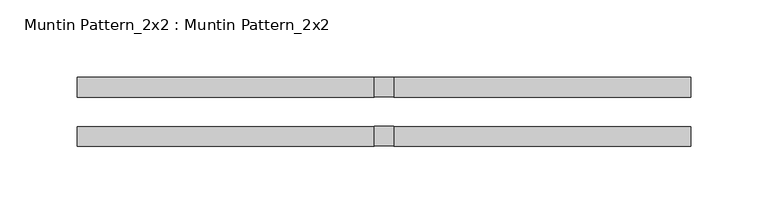
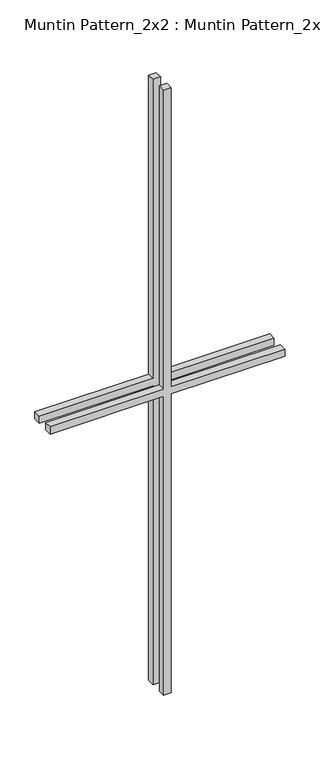
"""IFC4 building model written with IfcOpenShell, lengths in millimetres: proxy geometry, Muntin Pattern_2x2 : Muntin Pattern_2x2."""

from ifc_helpers import new_model, si_unit, frame, origin, place, context, project, spatial, polyline, outline, extrude, source, transform, mapped, element, save


def muntin_pattern_2x2_muntin_pattern_2x2_63e5058f(model_context):
    return source(origin(), model_context, "Body", "SweptSolid", [
        extrude(outline(polyline([(546.1, -6.35), (546.1, -198.4375), (533.4, -198.4375), (533.4, -6.35), (0.0, -6.35), (0.0, 6.35), (533.4, 6.35), (533.4, 198.4375), (546.1, 198.4375), (546.1, 6.35), (1079.5, 6.35), (1079.5, -6.35), (546.1, -6.35)])), frame((0.0, 9.525, 0.0), z_axis=(0.0, 1.0, 0.0), x_axis=(0.0, 0.0, 1.0)), (0.0, 0.0, 1.0), 12.7),
        extrude(outline(polyline([(546.1, -6.35), (546.1, -198.4375), (533.4, -198.4375), (533.4, -6.35), (0.0, -6.35), (0.0, 6.35), (533.4, 6.35), (533.4, 198.4375), (546.1, 198.4375), (546.1, 6.35), (1079.5, 6.35), (1079.5, -6.35), (546.1, -6.35)])), frame((0.0, -22.225, 0.0), z_axis=(0.0, 1.0, 0.0), x_axis=(0.0, 0.0, 1.0)), (0.0, 0.0, 1.0), 12.7),
    ])


if __name__ == "__main__":
    model = new_model("IFC4")
    model_context = context("Model", 3, world=origin())
    ifc_project = project(units=[si_unit("LENGTHUNIT", "METRE", prefix="MILLI")], contexts=[model_context])
    site = spatial("IfcSite", under=ifc_project)
    building = spatial("IfcBuilding", under=site)
    placement = place(None, origin())
    muntin_pattern_2x2_muntin_pattern_2x2_shape = muntin_pattern_2x2_muntin_pattern_2x2_63e5058f(model_context)
    element("IfcBuildingElementProxy", 1, Name="Muntin Pattern_2x2 : Muntin Pattern_2x2", ObjectType="Muntin Pattern_2x2 : Muntin Pattern_2x2", at=placement, inside=building, context=model_context, shape_type="MappedRepresentation", body=[
        mapped(muntin_pattern_2x2_muntin_pattern_2x2_shape, transform((0.0, 0.0, 0.0), x_axis=(1.0, 0.0, 0.0), y_axis=(0.0, 1.0, 0.0), z_axis=(0.0, 0.0, 1.0))),
    ])
    save(model, "model.ifc")

# Revit data of these elements
# Type "Muntin Pattern_2x2 : Muntin Pattern_2x2"
#   Width [instance default] = 4' - 0"
#   Thickness = 0' - 0 1/2"
#   Height [instance default] = 4' - 0"
#   Distance = 0' - 0 3/4"
#   Interior Material [instance default] = none
#   Exterior Material [instance default] = none
#   Default Elevation = 0
# Element 1 (IfcBuildingElementProxy, "Muntin Pattern_2x2 : Muntin Pattern_2x2")
#   Width = 1' - 3 5/8"
#   Height = 3' - 6 1/2"
#   Interior Material = Wood - Stained
#   Exterior Material = Clad - White
#   Materials on its faces: "Clad - White", "Wood - Stained"
# Materials
#   "Clad - White": class "Wood", colour RGB 242 242 238, transparency 0, Cost = 0
#   "Wood - Stained": class "Wood", colour RGB 224 178 126, transparency 0, Cost = 0
